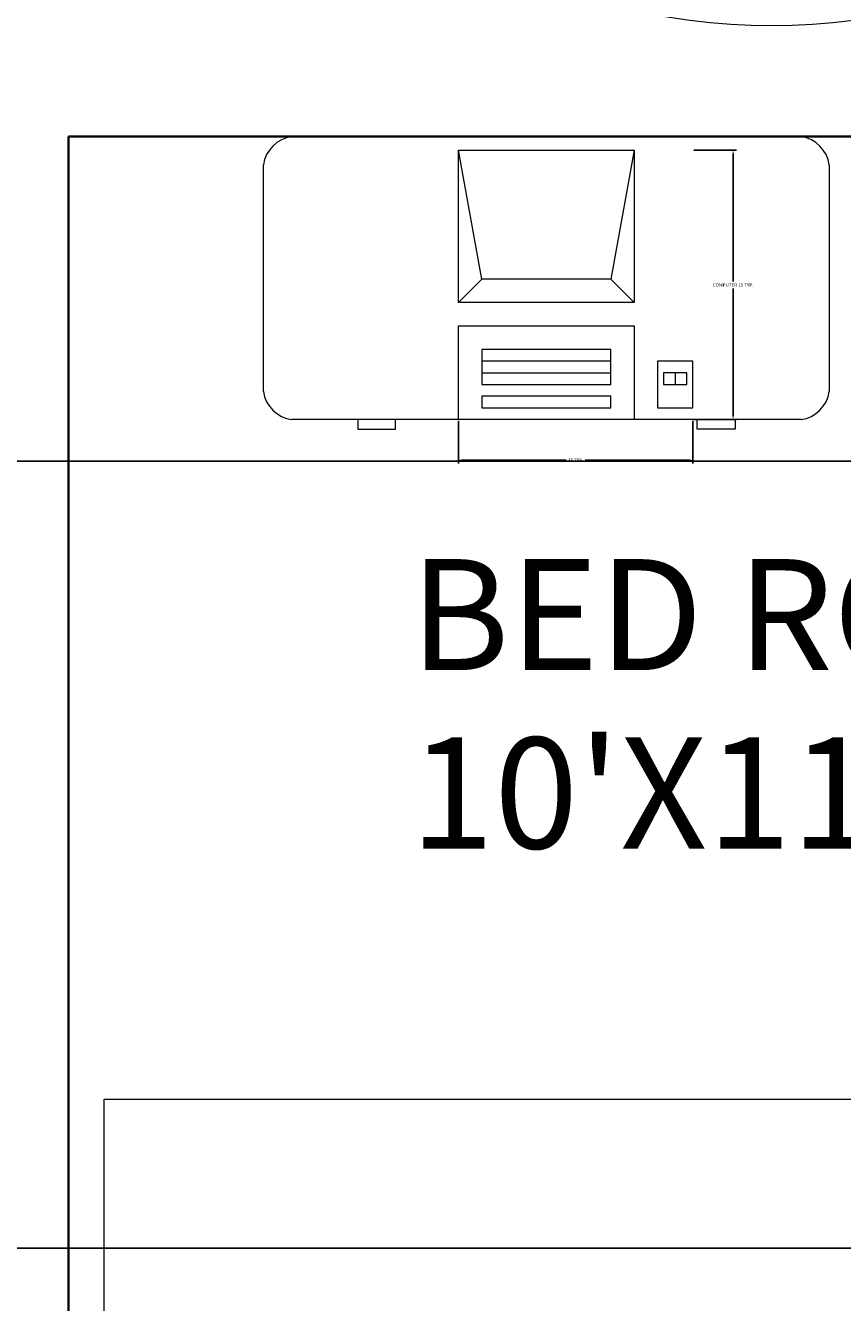
# Model space of a CAD drawing. Units: inches. Extents: x 4159 to 4826, y 299 to 1026.
# Tile 30 of 37: x 4546 to 4590, y 470 to 539. Entities that reach past the tile are written whole.
import ezdxf

# ---------------------------------------------------------------- set-up
doc = ezdxf.new("R2010")
doc.units = ezdxf.units.IN
for name, color, linetype, lineweight in [('A-ANNO-DIMS', 2, 'Continuous', 18), ('A-AREA-IDEN', 7, 'Continuous', 18), ('A-EQPM', 8, 'Continuous', 13), ('A-FURN', 8, 'Continuous', 18), ('A-WALL', 7, 'Continuous', 35)]:
    doc.layers.add(name, color=color, linetype=linetype, lineweight=lineweight)
doc.styles.get("Standard").update_dxf_attribs({"font": 'arial.ttf'})
doc.dimstyles.get("Standard").update_dxf_attribs({"dimtxt": 0.18, "dimasz": 0.18, "dimexe": 0.18, "dimexo": 0.0625, "dimgap": 0.09, "dimtad": 0, "dimtih": 1, "dimtoh": 1, "dimdec": 4, "dimzin": 0, "dimdsep": 46, "dimtxsty": 'Standard', "dimcen": 0.09, "dimadec": 0, "dimazin": 0, "dimtfac": 1, "dimtdec": 4, "dimtofl": 0, "dimtmove": 0, "dimatfit": 3, "dimfxl": 1, "dimtolj": 1, "dimtzin": 0, "dimarcsym": 0})

# ---------------------------------------------------------------- blocks, each defined once
blk = doc.blocks.new('Bed - Queen')
for p, q in [((59.99999, 0), (59.99999, -80.00003)), ((59.99999, -80.00003), (0, -80.00003))]:
    blk.add_line(p, q)
blk = doc.blocks.new('Sofa - Roundback Loveseat 5 ft.')
for p, q in [((0, -32.44198), (0, -5.99998)), ((-24, -33.99998), (-24, -11.46958)), ((24.00004, -33.99998), (24.00004, -11.46958)), ((-23.9998, -13.38178), (23.99986, -13.38178)), ((-24, -32.44198), (24.00004, -32.44198))]:
    blk.add_line(p, q)
for points in [[(-24, -33.99998), (-30, -33.99998), (-30, -7.99998)], [(30.00004, -7.99998), (30.00004, -33.99998), (24.00004, -33.99998)]]:
    blk.add_lwpolyline(points)
for centre, radius, start, end in [((0, -60.24998), 60.24998, 60.13715, 119.8628), ((0, -61.38438), 55.38444, 64.32083, 115.6792)]:
    blk.add_arc(centre, radius, start, end)
blk = doc.blocks.new('Desk - 30 x 60 in.')
for p, q in [((-26.999995, 0), (26.999995, 0)), ((-29.999995, -27), (-29.999995, -3)), ((29.999995, -3), (29.999995, -27)), ((26.999995, -30), (-26.999995, -30)), ((-20.000005, -30), (-20.000005, -31)), ((-20.000005, -31), (-16.000005, -31)), ((-16.000005, -31), (-16.000005, -30)), ((15.999995, -31), (15.999995, -30)), ((19.999995, -31), (15.999995, -31)), ((19.999995, -30), (19.999995, -31))]:
    blk.add_line(p, q)
for centre, start, end in [((-26.499995, -3.5), 98.1301, 171.8699), ((26.499995, -3.5), 8.130102, 81.8699), ((-26.499995, -26.5), 188.1301, 261.8699), ((26.499995, -26.5), 278.1301, 351.8699)]:
    blk.add_arc(centre, 3.535534, start, end)
blk = doc.blocks.new('Computer Terminal')
for p, q in [((-10, 11.5), (5, 11.5)), ((-8, 0.5), (-10, 11.5)), ((-10, -1.5), (-10, 11.5)), ((5, 11.5), (3, 0.5)), ((5, 11.5), (5, -1.5)), ((-10, -1.5), (-8, 0.5)), ((3, 0.5), (-8, 0.5)), ((3, 0.5), (5, -1.5)), ((5, -1.5), (-10, -1.5)), ((-10, -11.5), (-10, -3.5)), ((-10, -3.5), (5, -3.5)), ((5, -3.5), (5, -11.5)), ((-8, -5.5), (-8, -8.5)), ((3, -5.5), (-8, -5.5)), ((3, -6.5), (-8, -6.5)), ((3, -8.5), (3, -5.5)), ((10, -6.5), (7, -6.5)), ((7, -6.5), (7, -10.5)), ((10, -10.5), (10, -6.5)), ((-8, -7.5), (3, -7.5)), ((9.5, -7.5), (7.5, -7.5)), ((7.5, -7.5), (7.5, -8.5)), ((8.5, -7.5), (8.5, -8.5)), ((9.5, -8.5), (9.5, -7.5)), ((-8, -8.5), (3, -8.5)), ((7.5, -8.5), (9.5, -8.5)), ((-8, -9.5), (-8, -10.5)), ((3, -9.5), (-8, -9.5)), ((3, -10.5), (3, -9.5)), ((-8, -10.5), (3, -10.5)), ((7, -10.5), (10, -10.5)), ((5, -11.5), (-10, -11.5))]:
    blk.add_line(p, q)
blk = doc.blocks.new('*D29')
at = {"layer": 'A-ANNO-DIMS', "color": 0, "lineweight": -2, "transparency": 16777216}
for p, q in [((4581.698, 532.513), (4583.999, 532.513)), ((4583.819, 532.333), (4583.819, 525.418)), ((4583.819, 518.138), (4583.819, 525.052)), ((4581.698, 517.958), (4583.999, 517.958))]:
    blk.add_line(p, q, dxfattribs=at)
at = {"layer": 'A-ANNO-DIMS', "color": 0, "transparency": 16777216}
for points in [[(4583.789, 532.333), (4583.849, 532.333), (4583.819, 532.513)], [(4583.789, 518.138), (4583.849, 518.138), (4583.819, 517.958)]]:
    blk.add_solid(points, dxfattribs=at)
at = {"layer": 'Defpoints', "color": 0, "transparency": 16777216}
for p in [(4581.635, 532.513), (4583.819, 532.513), (4581.635, 517.958)]:
    blk.add_point(p, dxfattribs=at)
at = {"layer": 'A-ANNO-DIMS', "color": 0, "transparency": 16777216, "insert": (4583.819, 525.235), "char_height": 0.18, "attachment_point": 5}
blk.add_mtext('\\A1;COMPUTER 15 TYP.', dxfattribs=at)
blk = doc.blocks.new('*D30')
at = {"layer": 'A-ANNO-DIMS', "color": 0, "lineweight": -2, "transparency": 16777216}
for p, q in [((4568.979, 517.895), (4568.979, 515.594)), ((4581.635, 517.895), (4581.635, 515.594)), ((4569.159, 515.774), (4574.787, 515.774)), ((4581.455, 515.774), (4575.827, 515.774))]:
    blk.add_line(p, q, dxfattribs=at)
at = {"layer": 'A-ANNO-DIMS', "color": 0, "transparency": 16777216}
for points in [[(4569.159, 515.804), (4569.159, 515.744), (4568.979, 515.774)], [(4581.455, 515.804), (4581.455, 515.744), (4581.635, 515.774)]]:
    blk.add_solid(points, dxfattribs=at)
at = {"layer": 'Defpoints', "color": 0, "transparency": 16777216}
for p in [(4568.979, 517.958), (4581.635, 517.958), (4581.635, 515.774)]:
    blk.add_point(p, dxfattribs=at)
at = {"layer": 'A-ANNO-DIMS', "color": 0, "transparency": 16777216, "insert": (4575.307, 515.774), "char_height": 0.18, "attachment_point": 5}
blk.add_mtext('\\A1;13 TYP.', dxfattribs=at)
blk = doc.blocks.new('*D54')
at = {"layer": 'A-ANNO-DIMS', "color": 0, "lineweight": -2, "transparency": 16777216}
for p, q in [((4501.373, 515.713), (4825.74, 515.713)), ((4825.56, 515.533), (4825.56, 494.636)), ((4825.56, 473.375), (4825.56, 494.272)), ((4541.952, 473.195), (4825.74, 473.195))]:
    blk.add_line(p, q, dxfattribs=at)
at = {"layer": 'A-ANNO-DIMS', "color": 0, "transparency": 16777216}
for points in [[(4825.53, 515.533), (4825.59, 515.533), (4825.56, 515.713)], [(4825.53, 473.375), (4825.59, 473.375), (4825.56, 473.195)]]:
    blk.add_solid(points, dxfattribs=at)
at = {"layer": 'Defpoints', "color": 0, "transparency": 16777216}
for p in [(4501.31, 515.713), (4825.56, 515.713), (4541.889, 473.195)]:
    blk.add_point(p, dxfattribs=at)
at = {"layer": 'A-ANNO-DIMS', "color": 0, "transparency": 16777216, "insert": (4825.56, 494.454), "char_height": 0.18, "attachment_point": 5}
blk.add_mtext('\\A1;42.52', dxfattribs=at)

msp = doc.modelspace()

# ---------------------------------------------------------------- linework, layer by layer
at = {"layer": 'A-WALL'}
for p, q in [((4615.31, 533.254), (4547.889, 533.254)), ((4615.31, 533.254), (4547.889, 533.254)), ((4547.889, 533.254), (4547.889, 401.254))]:
    msp.add_line(p, q, dxfattribs=at)

# ---------------------------------------------------------------- block references
at = {"layer": 'A-EQPM', "xscale": 0.6328414688201627, "yscale": 0.6328414688201627, "zscale": 0.6328414688201627}
msp.add_blockref('Computer Terminal', (4575.307, 525.235), dxfattribs=at)
at = {"layer": 'A-FURN', "xscale": 0.5700533147329089, "yscale": 0.5700533147329089, "zscale": 0.5700533147329089, "rotation": 180}
msp.add_blockref('Sofa - Roundback Loveseat 5 ft.', (4585.903, 539.254), dxfattribs=at)
at = {"layer": 'A-FURN', "xscale": 0.5098837128326598, "yscale": 0.5098837128326598, "zscale": 0.5098837128326598}
msp.add_blockref('Desk - 30 x 60 in.', (4573.725, 533.254), dxfattribs=at)
at = {"layer": 'A-FURN', "rotation": 180}
msp.add_blockref('Bed - Queen', (4609.814, 401.246), dxfattribs=at)

# ---------------------------------------------------------------- texts
at = {"layer": 'A-AREA-IDEN'}
for s, p in [('BED ROOM', (4566.36, 504.422)), ("10'X11'", (4566.36, 494.784))]:
    msp.add_text(s, height=6, dxfattribs=at).set_placement(p)

# ---------------------------------------------------------------- dimensions: what is measured, and where the dimension line sits
at = {"layer": 'A-ANNO-DIMS'}
dim = msp.add_linear_dim(base=(4583.819, 532.513), p1=(4581.635, 517.958), p2=(4581.635, 532.513), angle=90, text='COMPUTER <> TYP.', dimstyle='Standard', override={"dimdec": 0, "dimlfac": 1, "dimrnd": 0, "dimzin": 0, "dimdsep": 46, "dimlunit": 2}, dxfattribs=at)
dim.commit()
dim.dimension.update_dxf_attribs({"geometry": '*D29', "text_midpoint": (4583.819, 525.235)})
dim = msp.add_linear_dim(base=(4581.635, 515.774), p1=(4568.979, 517.958), p2=(4581.635, 517.958), text='<> TYP.', dimstyle='Standard', override={"dimdec": 0, "dimlfac": 1, "dimrnd": 0, "dimzin": 0, "dimdsep": 46, "dimlunit": 2}, dxfattribs=at)
dim.commit()
dim.dimension.update_dxf_attribs({"geometry": '*D30', "text_midpoint": (4575.307, 515.774)})
dim = msp.add_linear_dim(base=(4825.56, 515.713), p1=(4541.889, 473.195), p2=(4501.31, 515.713), angle=90, dimstyle='Standard', override={"dimdec": 2, "dimlfac": 1, "dimrnd": 0, "dimzin": 0, "dimdsep": 46, "dimlunit": 2}, dxfattribs=at)
dim.commit()
dim.dimension.update_dxf_attribs({"geometry": '*D54', "text_midpoint": (4825.56, 494.454)})

doc.saveas('drawing.dxf')
